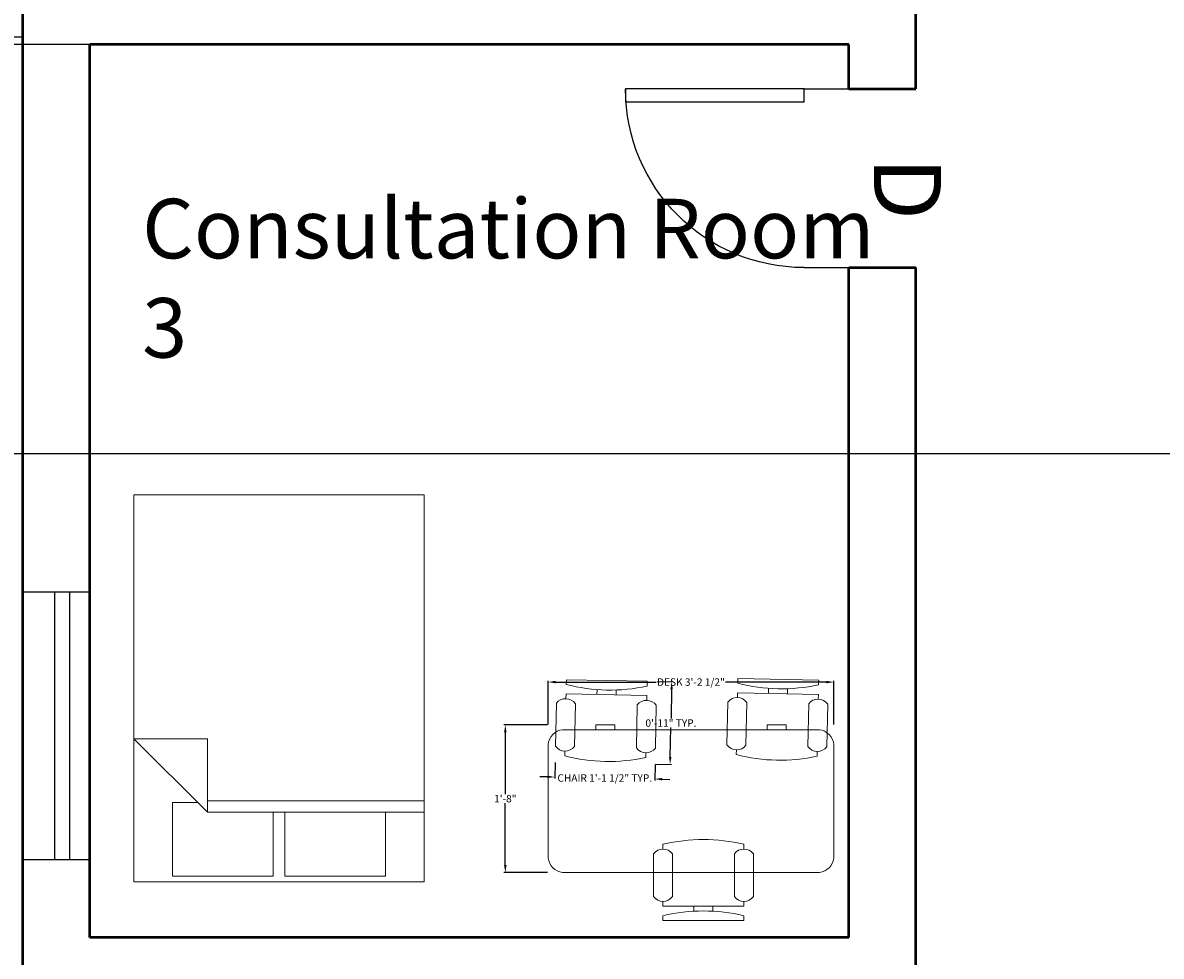
# Model space of a CAD drawing. Units: inches. Extents: x -364 to 705, y -52 to 1250.
# Tile 8 of 34: x 29 to 182, y 455 to 580. Entities that reach past the tile are written whole.
import ezdxf

# ---------------------------------------------------------------- set-up
doc = ezdxf.new("R2010")
doc.units = ezdxf.units.IN
doc.header["$MEASUREMENT"] = 0
for name, color, linetype, lineweight in [('A-ANNO-DIMS', 4, 'Continuous', 18), ('A-ANNO-IDEN', 1, 'Continuous', 18), ('A-AREA-IDEN', 3, 'Continuous', 18), ('A-DOOR', 1, 'Continuous', 25), ('A-FURN', 8, 'Continuous', 18), ('A-GLAZ', 4, 'Continuous', 25), ('A-WALL', 41, 'Continuous', 50)]:
    doc.layers.add(name, color=color, linetype=linetype, lineweight=lineweight)
doc.styles.get("Standard").update_dxf_attribs({"font": 'arial.ttf'})
doc.dimstyles.get("Standard").update_dxf_attribs({"dimtxt": 1, "dimasz": 1, "dimexe": 0.18, "dimexo": 0.0625, "dimgap": 0.09, "dimtad": 0, "dimtih": 1, "dimtoh": 1, "dimdec": 0, "dimzin": 0, "dimdsep": 46, "dimlunit": 3, "dimtxsty": 'Standard', "dimcen": 0.09, "dimadec": 0, "dimazin": 0, "dimtfac": 1, "dimtdec": 0, "dimtofl": 0, "dimtmove": 0, "dimatfit": 3, "dimfxl": 1, "dimtolj": 1, "dimtzin": 0, "dimarcsym": 0})

# ---------------------------------------------------------------- blocks, each defined once
blk = doc.blocks.new('Chair - Desk')
for p, q in [((-8.5, 0), (-8.5, -1)), ((-8.5, 0), (8.5, 0)), ((8.5, 0), (8.5, -1)), ((-2, -3), (-2, -1.9355)), ((2, -1.9576), (2, -3)), ((-8.5, -3), (-8.5, -4)), ((-8.5, -3), (8.5, -3)), ((8.5, -3), (8.5, -4)), ((-10.5, -5), (-10.5, -14)), ((-6.5, -14), (-6.5, -5)), ((6.5, -5), (6.5, -14)), ((10.5, -14), (10.5, -5)), ((-8.5, -15), (-8.5, -16)), ((8.5, -15), (8.5, -16))]:
    blk.add_line(p, q)
for centre, radius, start, end in [((0, 34.625), 36.625, 256.5803, 283.4197), ((-8.5, -6.5), 2.5, 36.8699, 143.1301), ((8.5, -6.5), 2.5, 36.8699, 143.1301), ((-8.5, -12.5), 2.5, 216.8699, 323.1301), ((8.5, -12.5), 2.5, 216.8699, 323.1301), ((0, 19.625), 36.625, 256.5803, 283.4197)]:
    blk.add_arc(centre, radius, start, end)
blk = doc.blocks.new('Desk - 30 x 60 in.')
for p, q in [((-26.999995, 0), (26.999995, 0)), ((-29.999995, -27), (-29.999995, -3)), ((29.999995, -3), (29.999995, -27)), ((26.999995, -30), (-26.999995, -30)), ((-20.000005, -30), (-20.000005, -31)), ((-20.000005, -31), (-16.000005, -31)), ((-16.000005, -31), (-16.000005, -30)), ((15.999995, -31), (15.999995, -30)), ((19.999995, -31), (15.999995, -31)), ((19.999995, -30), (19.999995, -31))]:
    blk.add_line(p, q)
for centre, start, end in [((-26.499995, -3.5), 98.1301, 171.8699), ((26.499995, -3.5), 8.130102, 81.8699), ((-26.499995, -26.5), 188.1301, 261.8699), ((26.499995, -26.5), 278.1301, 351.8699)]:
    blk.add_arc(centre, 3.535534, start, end)
blk = doc.blocks.new('Bed - Queen')
for p, q in [((0, -80.00003), (0, 0)), ((0, 0), (59.99999, 0)), ((59.99999, 0), (59.99999, -80.00003)), ((7.99999, -1.2), (28.79998, -1.2)), ((7.99999, -14.4), (7.99999, -1.2)), ((28.79998, -1.2), (28.79998, -14.4)), ((31.19999, -1.2), (51.99999, -1.2)), ((31.19999, -14.4), (31.19999, -1.2)), ((51.99999, -1.2), (51.99999, -16.4)), ((0, -14.4), (44.8, -14.4)), ((59.99999, -29.6), (44.8, -14.4)), ((44.8, -14.4), (44.8, -29.6)), ((51.99999, -16.4), (46.79936, -16.4)), ((44.8, -16.8), (0, -16.8)), ((44.8, -29.6), (59.99999, -29.6)), ((59.99999, -80.00003), (0, -80.00003))]:
    blk.add_line(p, q)
blk = doc.blocks.new('*U16')
for p, q in [((-24, 0), (-24, 6)), ((0, 0), (0, 6))]:
    blk.add_line(p, q)
blk.add_lwpolyline([(0, 0), (0, -24), (-1.75, -24), (-1.75, 0)], close=True)
blk.add_arc((0, 0), 24, 180, 270)
blk = doc.blocks.new('*D19')
at = {"layer": 'A-ANNO-DIMS', "color": 0, "lineweight": -2, "transparency": 16777216}
for p, q in [((28.52, 986.11), (-248.33, 986.11)), ((-248.15, 985.11), (-248.15, 574.22)), ((-248.15, 149.87), (-248.15, 560.77)), ((28.52, 148.87), (-248.33, 148.87))]:
    blk.add_line(p, q, dxfattribs=at)
at = {"layer": 'A-ANNO-DIMS', "color": 0, "transparency": 16777216}
for points in [[(-248.32, 985.11), (-247.99, 985.11), (-248.15, 986.11)], [(-248.32, 149.87), (-247.99, 149.87), (-248.15, 148.87)]]:
    blk.add_solid(points, dxfattribs=at)
at = {"layer": 'Defpoints', "color": 0, "transparency": 16777216}
for p in [(28.58, 986.11), (-248.15, 148.87), (28.58, 148.87)]:
    blk.add_point(p, dxfattribs=at)
at = {"layer": 'A-ANNO-DIMS', "color": 0, "transparency": 16777216, "insert": (-248.15, 567.49), "char_height": 1, "attachment_point": 5}
blk.add_mtext('\\A1;{\\H13x;69\'-9"}', dxfattribs=at)
blk = doc.blocks.new('*D30')
at = {"layer": 'A-ANNO-DIMS', "color": 0, "lineweight": -2, "transparency": 16777216}
for p, q in [((28.52, 578.1), (-188.97, 578.1)), ((-188.79, 577.1), (-188.79, 521.83)), ((-188.79, 453.11), (-188.79, 508.38)), ((28.52, 452.11), (-188.97, 452.11))]:
    blk.add_line(p, q, dxfattribs=at)
at = {"layer": 'A-ANNO-DIMS', "color": 0, "transparency": 16777216}
for points in [[(-188.96, 577.1), (-188.63, 577.1), (-188.79, 578.1)], [(-188.96, 453.11), (-188.63, 453.11), (-188.79, 452.11)]]:
    blk.add_solid(points, dxfattribs=at)
at = {"layer": 'Defpoints', "color": 0, "transparency": 16777216}
for p in [(-188.79, 578.1), (28.58, 578.1), (28.58, 452.11)]:
    blk.add_point(p, dxfattribs=at)
at = {"layer": 'A-ANNO-DIMS', "color": 0, "transparency": 16777216, "insert": (-188.79, 515.11), "char_height": 1, "attachment_point": 5}
blk.add_mtext('\\A1;{\\H13x;10\'-6"}', dxfattribs=at)
blk = doc.blocks.new('*D31')
at = {"layer": 'A-ANNO-DIMS', "color": 0, "lineweight": -2, "transparency": 16777216}
for p, q in [((37.52, 706.11), (-205.07, 706.11)), ((-204.89, 705.11), (-204.89, 648.34)), ((-204.89, 578.11), (-204.89, 634.89)), ((37.52, 577.11), (-205.07, 577.11))]:
    blk.add_line(p, q, dxfattribs=at)
at = {"layer": 'A-ANNO-DIMS', "color": 0, "transparency": 16777216}
for points in [[(-205.06, 705.11), (-204.73, 705.11), (-204.89, 706.11)], [(-205.06, 578.11), (-204.73, 578.11), (-204.89, 577.11)]]:
    blk.add_solid(points, dxfattribs=at)
at = {"layer": 'Defpoints', "color": 0, "transparency": 16777216}
for p in [(37.58, 706.11), (-204.89, 577.11), (37.58, 577.11)]:
    blk.add_point(p, dxfattribs=at)
at = {"layer": 'A-ANNO-DIMS', "color": 0, "transparency": 16777216, "insert": (-204.89, 641.61), "char_height": 1, "attachment_point": 5}
blk.add_mtext('\\A1;{\\H13x;10\'-9"}', dxfattribs=at)
blk = doc.blocks.new('WIN-36-DOUBLE-LINE')
for p, q in [((4.27, 36), (4.27, 0)), ((6.27, 36), (6.27, 0))]:
    blk.add_line(p, q)
blk.add_lwpolyline([(9, 36), (9, 0), (0, 0), (0, 36)], close=True)
blk = doc.blocks.new('*D44')
at = {"layer": 'A-ANNO-DIMS', "color": 0, "lineweight": -2, "transparency": 16777216}
for p, q in [((100.12, 480.64), (100.08, 478.51)), ((113.56, 480.37), (113.51, 478.24)), ((99.08, 478.71), (98.09, 478.73)), ((114.52, 478.4), (115.52, 478.38))]:
    blk.add_line(p, q, dxfattribs=at)
at = {"layer": 'A-ANNO-DIMS', "color": 0, "transparency": 16777216}
for points in [[(99.09, 478.88), (99.08, 478.55), (100.08, 478.69)], [(114.52, 478.57), (114.51, 478.23), (113.52, 478.42)]]:
    blk.add_solid(points, dxfattribs=at)
at = {"layer": 'Defpoints', "color": 0, "transparency": 16777216}
for p in [(100.13, 480.71), (113.56, 480.44), (113.52, 478.42)]:
    blk.add_point(p, dxfattribs=at)
at = {"layer": 'A-ANNO-DIMS', "color": 0, "transparency": 16777216, "insert": (106.8, 478.56), "char_height": 1, "attachment_point": 5}
blk.add_mtext('\\A1;CHAIR 1\'-1 1/2" TYP.', dxfattribs=at)
blk = doc.blocks.new('*D45')
at = {"layer": 'A-ANNO-DIMS', "color": 0, "lineweight": -2, "transparency": 16777216}
for p, q in [((113.84, 491.52), (115.98, 491.48)), ((115.78, 490.48), (115.7, 486.54)), ((115.59, 481.39), (115.67, 485.34)), ((113.62, 480.43), (115.75, 480.39))]:
    blk.add_line(p, q, dxfattribs=at)
at = {"layer": 'A-ANNO-DIMS', "color": 0, "transparency": 16777216}
for points in [[(115.61, 490.48), (115.94, 490.48), (115.8, 491.48)], [(115.43, 481.4), (115.76, 481.39), (115.57, 480.39)]]:
    blk.add_solid(points, dxfattribs=at)
at = {"layer": 'Defpoints', "color": 0, "transparency": 16777216}
for p in [(113.78, 491.52), (115.8, 491.48), (113.56, 480.44)]:
    blk.add_point(p, dxfattribs=at)
at = {"layer": 'A-ANNO-DIMS', "color": 0, "transparency": 16777216, "insert": (115.69, 485.94), "char_height": 1, "attachment_point": 5}
blk.add_mtext('\\A1;0\'-11" TYP.', dxfattribs=at)
blk = doc.blocks.new('*D56')
at = {"layer": 'A-ANNO-DIMS', "color": 0, "lineweight": -2, "transparency": 16777216}
for p, q in [((99.19, 485.75), (99.19, 491.63)), ((100.19, 491.45), (113.72, 491.45)), ((136.57, 491.45), (123.04, 491.45)), ((137.57, 485.75), (137.57, 491.63))]:
    blk.add_line(p, q, dxfattribs=at)
at = {"layer": 'A-ANNO-DIMS', "color": 0, "transparency": 16777216}
for points in [[(100.19, 491.62), (100.19, 491.28), (99.19, 491.45)], [(136.57, 491.62), (136.57, 491.28), (137.57, 491.45)]]:
    blk.add_solid(points, dxfattribs=at)
at = {"layer": 'Defpoints', "color": 0, "transparency": 16777216}
for p in [(99.19, 491.45), (99.19, 485.69), (137.57, 485.69)]:
    blk.add_point(p, dxfattribs=at)
at = {"layer": 'A-ANNO-DIMS', "color": 0, "transparency": 16777216, "insert": (118.38, 491.45), "char_height": 1, "attachment_point": 5}
blk.add_mtext('\\A1;DESK 3\'-2 1/2"', dxfattribs=at)
blk = doc.blocks.new('*D57')
at = {"layer": 'A-ANNO-DIMS', "color": 0, "lineweight": -2, "transparency": 16777216}
for p, q in [((99.12, 485.69), (93.25, 485.69)), ((93.43, 484.69), (93.43, 476.38)), ((93.43, 466.86), (93.43, 475.18)), ((99.12, 465.86), (93.25, 465.86))]:
    blk.add_line(p, q, dxfattribs=at)
at = {"layer": 'A-ANNO-DIMS', "color": 0, "transparency": 16777216}
for points in [[(93.26, 484.69), (93.6, 484.69), (93.43, 485.69)], [(93.26, 466.86), (93.6, 466.86), (93.43, 465.86)]]:
    blk.add_solid(points, dxfattribs=at)
at = {"layer": 'Defpoints', "color": 0, "transparency": 16777216}
for p in [(99.19, 485.69), (93.43, 465.86), (99.19, 465.86)]:
    blk.add_point(p, dxfattribs=at)
at = {"layer": 'A-ANNO-DIMS', "color": 0, "transparency": 16777216, "insert": (93.43, 475.78), "char_height": 1, "attachment_point": 5}
blk.add_mtext('\\A1;1\'-8"', dxfattribs=at)
blk = doc.blocks.new('*D98')
at = {"layer": 'A-ANNO-DIMS', "color": 0, "lineweight": -2, "transparency": 16777216}
for p, q in [((358.52, 642.11), (-126.85, 642.11)), ((-126.67, 641.11), (-126.67, 582.72)), ((-126.67, 523.11), (-126.67, 581.51)), ((358.52, 522.11), (-126.85, 522.11))]:
    blk.add_line(p, q, dxfattribs=at)
at = {"layer": 'A-ANNO-DIMS', "color": 0, "transparency": 16777216}
for points in [[(-126.84, 641.11), (-126.5, 641.11), (-126.67, 642.11)], [(-126.84, 523.11), (-126.5, 523.11), (-126.67, 522.11)]]:
    blk.add_solid(points, dxfattribs=at)
at = {"layer": 'Defpoints', "color": 0, "transparency": 16777216}
for p in [(-126.67, 642.11), (358.58, 642.11), (358.58, 522.11)]:
    blk.add_point(p, dxfattribs=at)
at = {"layer": 'A-ANNO-DIMS', "color": 0, "transparency": 16777216, "insert": (-126.67, 582.11), "char_height": 1, "attachment_point": 5}
blk.add_mtext('\\A1;10\'-0"', dxfattribs=at)

msp = doc.modelspace()

# ---------------------------------------------------------------- linework, layer by layer
at = {"layer": 'A-WALL'}
for p, q in [((28.58, 11.11), (28.58, 986.11)), ((148.58, 571.14), (148.58, 676.98)), ((139.58, 577.11), (37.58, 577.11)), ((37.58, 457.11), (37.58, 577.11)), ((139.58, 571.14), (139.58, 577.11)), ((139.58, 571.14), (139.58, 576.14)), ((139.58, 571.14), (148.58, 571.14)), ((139.58, 457.11), (139.58, 547.14)), ((139.58, 547.14), (148.58, 547.14)), ((148.58, 446.97), (148.58, 547.14)), ((139.58, 457.11), (37.58, 457.11))]:
    msp.add_line(p, q, dxfattribs=at)

# ---------------------------------------------------------------- block references
at = {"layer": 'A-DOOR', "xscale": -1, "rotation": 270.0000000000011}
msp.add_blockref('*U16', (133.58, 571.14), dxfattribs=at)
at = {"layer": 'A-FURN'}
for name, p, xscale, yscale, zscale, rotation in [('Bed - Queen', (82.52, 464.59), 0.6500148169160638, 0.6500148169160638, 0.6500148169160638, 180), ('Chair - Desk', (107.07, 491.66), 0.6397732151205352, 0.6397732151205352, 0.6397732151205352, 358.8399543093713), ('Chair - Desk', (130.11, 491.83), 0.6397732151205352, 0.6397732151205352, 0.6397732151205352, 358.8399543093713), ('Desk - 30 x 60 in.', (118.38, 465.86), 0.6397732151205352, 0.6397732151205352, 0.6397732151205352, 180), ('Chair - Desk', (120.06, 459.42), 0.6397732151205352, 0.6397732151205352, 0.6397732151205352, 180)]:
    msp.add_blockref(name, p, dxfattribs=dict(at, xscale=xscale, yscale=yscale, zscale=zscale, rotation=rotation))
at = {"layer": 'A-GLAZ'}
msp.add_blockref('WIN-36-DOUBLE-LINE', (28.59, 467.58), dxfattribs=at)

# ---------------------------------------------------------------- texts
at = {"layer": 'A-ANNO-IDEN', "insert": (151.98, 561.97), "char_height": 9, "attachment_point": 1, "rotation": 270}
msp.add_mtext_dynamic_manual_height_columns('D', width=16.916, gutter_width=1, heights=[0], dxfattribs=at)
at = {"layer": 'A-AREA-IDEN', "insert": (44.62, 556.38), "char_height": 8, "attachment_point": 1}
msp.add_mtext_dynamic_manual_height_columns('Consultation Room 3', width=101.5397, gutter_width=1, heights=[0], dxfattribs=at)

# ---------------------------------------------------------------- dimensions: what is measured, and where the dimension line sits
at = {"layer": 'A-ANNO-DIMS'}
for base, p1, p2, angle, text, override, picture, middle in [((-248.15, 148.87), (28.58, 986.11), (28.58, 148.87), 90, '{\\H13x;<>}', {"dimclrd": 0, "dimclre": 0, "dimclrt": 0}, '*D19', (-248.15, 567.49)), ((-204.89, 577.11), (37.58, 706.11), (37.58, 577.11), 90, '{\\H13x;<>}', {"dimclrd": 0, "dimclre": 0, "dimclrt": 0}, '*D31', (-204.89, 641.61)), ((-188.79, 578.1), (28.58, 452.11), (28.58, 578.1), 90, '{\\H13x;<>}', {"dimclrd": 0, "dimclre": 0, "dimclrt": 0}, '*D30', (-188.79, 515.11)), ((99.19, 491.45), (137.57, 485.69), (99.19, 485.69), 180, 'DESK <>', {"dimdec": 1, "dimlfac": 1, "dimrnd": 0, "dimzin": 1, "dimdsep": 46, "dimlunit": 4, "dimfrac": 2}, '*D56', (118.38, 491.45)), ((115.8, 491.48), (113.56, 480.44), (113.78, 491.52), 88.84, '<> TYP.', {"dimdec": 1, "dimlfac": 1, "dimrnd": 0, "dimzin": 1, "dimdsep": 46, "dimlunit": 4, "dimfrac": 2}, '*D45', (115.69, 485.94)), ((113.52, 478.42), (100.13, 480.71), (113.56, 480.44), 358.84, 'CHAIR <> TYP.', {"dimdec": 1, "dimlfac": 1, "dimrnd": 0, "dimzin": 1, "dimdsep": 46, "dimlunit": 4, "dimfrac": 2}, '*D44', (106.8, 478.56))]:
    dim = msp.add_linear_dim(base=base, p1=p1, p2=p2, angle=angle, text=text, dimstyle='Standard', override=override, dxfattribs=at)
    dim.commit()
    dim.dimension.update_dxf_attribs({"geometry": picture, "text_midpoint": middle})
for base, p1, p2, angle, picture, middle in [((-126.67, 642.11), (358.58, 522.11), (358.58, 642.11), 90, '*D98', (-126.67, 582.11)), ((93.43, 465.86), (99.19, 485.69), (99.19, 465.86), 270, '*D57', (93.43, 475.78))]:
    dim = msp.add_linear_dim(base=base, p1=p1, p2=p2, angle=angle, dimstyle='Standard', override={"dimdec": 1, "dimlfac": 1, "dimrnd": 0, "dimzin": 1, "dimdsep": 46, "dimlunit": 4, "dimfrac": 2}, dxfattribs=at)
    dim.commit()
    dim.dimension.update_dxf_attribs({"geometry": picture, "text_midpoint": middle})

doc.saveas('drawing.dxf')
